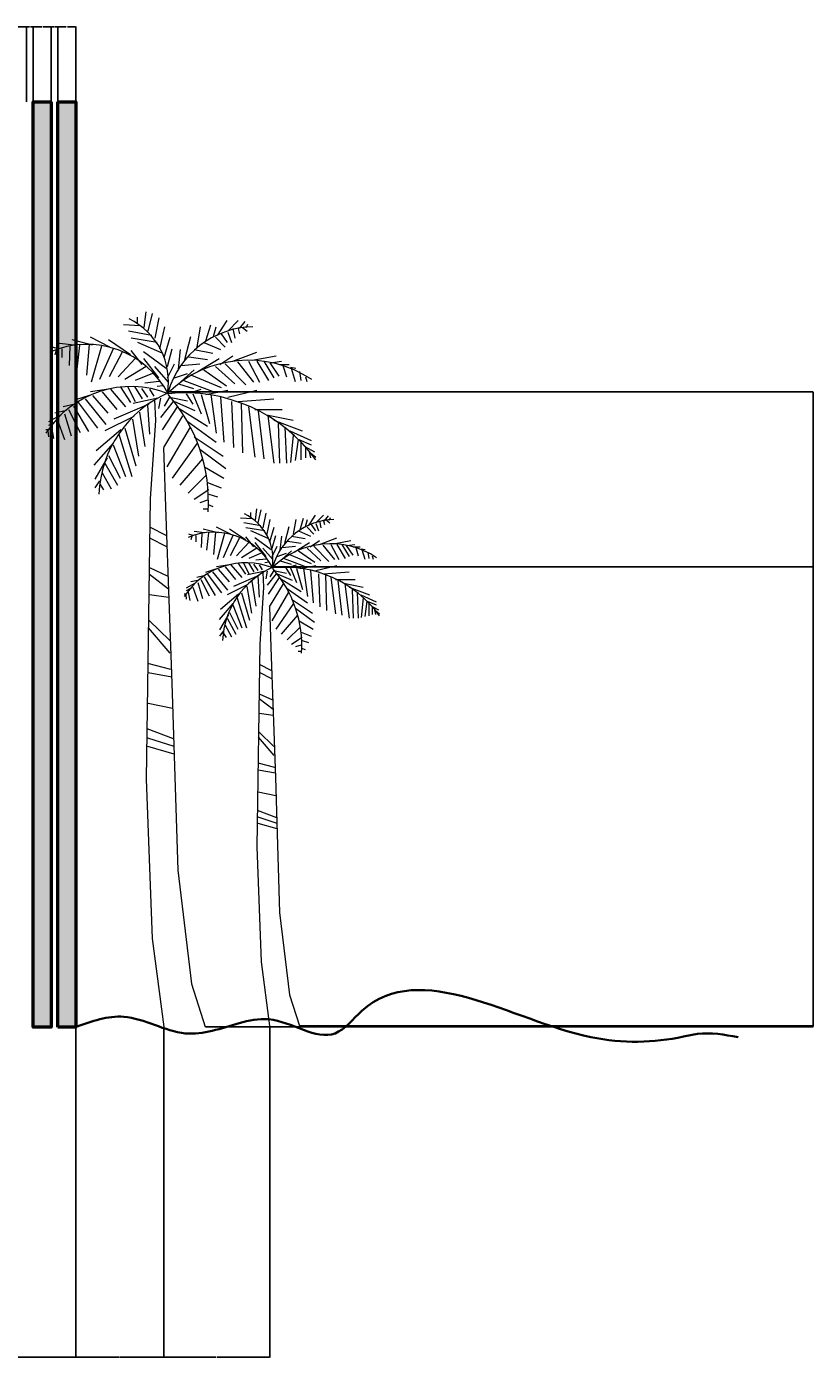
# Model space of a CAD drawing. Units: inches. Extents: x -97 to 1206, y -378 to 680.
# Tile 6 of 6: x 581 to 1206, y -378 to 680. Entities that reach past the tile are written whole.
import ezdxf

# ---------------------------------------------------------------- set-up
doc = ezdxf.new("R2010")
doc.units = ezdxf.units.IN
doc.header["$MEASUREMENT"] = 0
for name, color, linetype, lineweight in [('A-ANNO-DIMS', 2, 'Continuous', 18), ('A-WALL', 7, 'Continuous', 50), ('A-WALL-PATT', 8, 'Continuous', 18), ('C-TOPO', 8, 'Continuous', 35), ('L-PLNT', 82, 'Continuous', 13)]:
    doc.layers.add(name, color=color, linetype=linetype, lineweight=lineweight)
doc.styles.get("Standard").update_dxf_attribs({"font": 'arial.ttf'})
doc.dimstyles.get("Standard").update_dxf_attribs({"dimtxt": 0.18, "dimasz": 0.18, "dimexe": 0.18, "dimexo": 0.0625, "dimgap": 0.09, "dimtad": 0, "dimtih": 1, "dimtoh": 1, "dimdec": 4, "dimzin": 0, "dimdsep": 46, "dimtxsty": 'Standard', "dimcen": 0.09, "dimadec": 0, "dimazin": 0, "dimtfac": 1, "dimtdec": 4, "dimtofl": 0, "dimtmove": 0, "dimatfit": 3, "dimfxl": 1, "dimtolj": 1, "dimtzin": 0, "dimarcsym": 0})
pattern_1 = [(228.0128, (-174.969, -144.922), (-376, -423), [6.3232, -625.9971]), (184.96974, (-179.199, -149.622), (564, 47), [10.8508, -1074.2285]), (132.51045, (-190.009, -150.562), (470, -517), [7.651, -757.4535]), (267.2737, (-208.339, -162.312), (47, 940), [9.8812, -978.2372]), (292.83365, (-208.809, -172.182), (-235, 564), [9.6893, -959.2405]), (357.2737, (-205.049, -181.112), (-940, 47), [9.8812, -978.2372]), (37.69424, (-195.179, -181.582), (-611, -470), [13.0674, -1293.6679]), (72.25533, (-184.839, -173.592), (329, 1034), [12.3369, -1221.3571]), (121.42957, (-181.079, -161.842), (-376, 611), [9.9146, -981.5514]), (175.23636, (-186.249, -153.382), (517, -47), [11.3191, -554.6358]), (222.39744, (-197.5289, -152.442), (-564, -517), [14.63806, -1449.1686]), (138.81407, (-161.809, -162.782), (-329, 282), [4.9961, -494.6207]), (171.46923, (-165.569, -159.492), (611, -94), [9.5051, -941.011]), (225, (-174.97, -158.082), (-5e-15, -47), [6.6468, -59.8213]), (203.1986, (-178.259, -152.442), (235, 94), [3.5794, -354.3619]), (291.8014, (-181.549, -153.852), (-47, 141), [5.062, -248.0407]), (30.96376, (-179.669, -158.552), (141, 94), [8.2217, -265.833]), (161.565, (-172.619, -154.322), (94, -47), [5.945, -142.682]), (16.38954, (-208.809, -153.852), (470, 141), [8.3284, -824.5137]), (70.34618, (-200.819, -151.502), (-188, -517), [6.9871, -691.7182]), (293.1986, (-172.619, -144.922), (-94, 235), [7.1588, -350.7825]), (343.61046, (-169.799, -151.502), (-470, 141), [8.3284, -824.5137]), (339.44395, (-208.809, -182.992), (-235, 94), [8.0314, -393.5368]), (294.77514, (-201.289, -185.812), (-235, 517), [6.7294, -666.2082]), (66.8014, (-172.149, -191.922), (94, 235), [7.1588, -350.7825]), (17.35402, (-169.329, -185.342), (-611, -188), [7.8787, -779.9849]), (69.44395, (-195.179, -191.922), (-94, -235), [4.0157, -397.5525]), (101.3099, (-174.969, -191.922), (-47, 188), [2.3965, -237.2574]), (165.9638, (-175.439, -189.572), (141, -47), [9.6893, -184.0967]), (186.009, (-184.839, -187.222), (470, 47), [8.9794, -888.9544]), (303.6901, (-179.669, -162.782), (-47, 94), [6.7784, -162.6825]), (353.15723, (-175.909, -168.422), (799, -94), [11.8343, -1171.5954]), (60.9454, (-164.159, -169.832), (-188, -329), [4.839, -479.0557]), (90, (-161.81, -165.6), (-47, 47), [2.82, -44.18]), (120.25644, (-185.779, -185.812), (188, -329), [6.5294, -646.4154]), (48.0128, (-189.069, -180.172), (376, 423), [12.6464, -619.674]), (0, (-180.61, -170.77), (47, 47), [12.22, -34.78]), (325.30485, (-168.389, -170.772), (470, -329), [7.4314, -735.7039]), (254.0546, (-162.279, -175.002), (-47, -188), [6.8433, -335.3219]), (207.64598, (-164.159, -181.582), (-893, -470), [11.1421, -1103.0653]), (175.42608, (-174.029, -186.752), (-611, 47), [11.7876, -1166.96645])]

# ---------------------------------------------------------------- blocks, each defined once
blk = doc.blocks.new('*U4')
for p, q in [((-7.5, 199.68), (-7.5, 197.946)), ((-5.567, 196.707), (-4.987, 201.167)), ((-4.407, 195.716), (-3.247, 200.672)), ((-2.474, 193.733), (-1.315, 199.433)), ((15.116, 194.477), (17.822, 198.689)), ((18.015, 195.716), (20.914, 198.689)), ((-6.727, 197.202), (-11.366, 197.45)), ((-3.441, 194.477), (-10.013, 195.716)), ((-1.121, 190.759), (0.232, 196.955)), ((9.317, 191.255), (10.283, 196.955)), ((11.829, 192.99), (13.182, 197.45)), ((13.956, 194.229), (14.729, 196.955)), ((16.082, 194.972), (17.822, 192.494)), ((18.015, 195.468), (18.981, 192.494)), ((19.368, 196.459), (19.948, 193.733)), ((20.914, 196.459), (21.301, 194.972)), ((21.301, 196.459), (22.847, 198.441)), ((22.074, 196.707), (23.427, 195.716)), ((23.234, 196.707), (23.62, 197.698)), ((-29.729, 190.759), (-31.469, 191.255)), ((-25.283, 191.751), (-29.342, 192.246)), ((-26.443, 191.503), (-26.636, 186.051)), ((-20.064, 191.751), (-25.863, 193.238)), ((-23.737, 191.751), (-24.51, 185.06)), ((-21.031, 191.998), (-21.804, 183.325)), ((-15.232, 191.255), (-20.644, 193.981)), ((-17.551, 191.503), (-20.451, 181.343)), ((-9.433, 189.025), (-15.618, 193.238)), ((-1.894, 192.494), (-9.24, 193.733)), ((-0.541, 189.52), (-7.307, 192.494)), ((0.038, 188.281), (1.778, 193.981)), ((5.837, 187.786), (7.577, 194.229)), ((11.25, 192.494), (15.889, 190.512)), ((14.536, 193.981), (17.242, 191.255)), ((-30.309, 190.512), (-30.695, 189.025)), ((-28.763, 190.759), (-28.763, 188.281)), ((-14.265, 190.759), (-18.131, 182.086)), ((-11.753, 189.768), (-15.425, 182.83)), ((-8.08, 188.034), (-12.912, 182.83)), ((-6.147, 186.299), (-9.24, 190.264)), ((-5.76, 190.016), (0.618, 185.308)), ((-5.76, 188.034), (-1.508, 182.582)), ((1.005, 185.803), (2.358, 190.759)), ((4.098, 185.06), (4.678, 190.512)), ((6.997, 188.529), (12.216, 187.786)), ((8.544, 190.512), (13.763, 189.52)), ((9.51, 184.317), (15.502, 188.034)), ((15.695, 186.299), (19.368, 188.777)), ((19.368, 187.29), (26.133, 189.768)), ((23.814, 187.29), (26.907, 181.343)), ((24.78, 187.538), (31.546, 188.777)), ((26.133, 187.29), (29.419, 181.838)), ((28.066, 187.29), (30.966, 182.582)), ((29.999, 186.795), (33.092, 187.29)), ((-4.987, 185.803), (-10.979, 182.086)), ((-3.247, 183.821), (-8.08, 181.838)), ((-2.668, 185.803), (1.198, 181.343)), ((1.005, 182.582), (2.938, 186.547)), ((2.938, 182.582), (6.61, 183.821)), ((4.871, 186.051), (10.09, 186.547)), ((4.871, 181.591), (8.544, 184.812)), ((11.25, 184.812), (17.628, 180.352)), ((14.536, 185.803), (19.948, 180.847)), ((17.242, 186.547), (23.041, 180.599)), ((20.721, 187.042), (25.167, 181.343)), ((29.806, 186.795), (32.319, 183.078)), ((32.512, 186.299), (35.218, 186.299)), ((33.479, 186.051), (34.445, 182.83)), ((35.605, 185.556), (37.151, 185.308)), ((35.798, 185.308), (36.958, 181.591)), ((38.118, 184.317), (38.504, 181.838)), ((-12.332, 180.104), (-9.433, 175.643)), ((-10.206, 180.104), (-8.08, 175.891)), ((-8.273, 180.104), (-6.147, 176.635)), ((-1.315, 181.591), (-5.374, 181.095)), ((-0.348, 180.352), (-1.894, 180.104)), ((4.098, 180.847), (8.35, 179.608)), ((5.644, 181.838), (13.569, 178.865)), ((7.77, 183.325), (16.082, 179.856)), ((39.857, 182.83), (40.244, 181.591)), ((-21.031, 177.626), (-24.897, 176.387)), ((-22.191, 176.635), (-16.391, 169.448)), ((-15.618, 179.36), (-20.644, 178.617)), ((-20.064, 177.626), (-15.812, 172.67)), ((-17.358, 178.617), (-13.299, 173.661)), ((-15.038, 179.36), (-10.786, 174.404)), ((-1.701, 176.882), (-8.66, 175.396)), ((-6.34, 179.608), (-4.6, 177.13)), ((-4.021, 179.36), (-2.861, 177.378)), ((-2.668, 176.387), (-2.376, 170.594)), ((-0.928, 176.882), (-1.508, 173.909)), ((1.585, 177.13), (0.038, 174.652)), ((1.585, 177.13), (6.61, 176.139)), ((6.224, 178.121), (8.157, 175.148)), ((7.384, 178.369), (10.476, 179.36)), ((8.157, 178.121), (10.476, 172.422)), ((10.476, 177.874), (12.796, 169.696)), ((11.829, 177.874), (18.015, 179.113)), ((13.182, 177.874), (14.729, 166.97)), ((15.889, 177.13), (16.855, 164.492)), ((18.015, 177.13), (26.133, 179.113)), ((20.914, 175.891), (30.966, 176.635)), ((-27.409, 173.413), (-30.695, 172.67)), ((-25.09, 175.148), (-28.376, 174.404)), ((-27.989, 172.422), (-26.056, 166.227)), ((-26.829, 173.661), (-23.544, 167.218)), ((-25.476, 174.652), (-21.224, 167.466)), ((-24.317, 175.891), (-18.711, 168.457)), ((-4.214, 175.148), (-14.072, 170.935)), ((-6.92, 172.917), (-5.374, 163.253)), ((-4.6, 174.9), (-4.021, 166.722)), ((2.551, 175.891), (-0.928, 171.431)), ((3.711, 174.404), (-0.541, 167.961)), ((2.938, 175.891), (8.737, 173.413)), ((4.291, 173.909), (12.216, 168.953)), ((18.981, 175.891), (19.561, 163.005)), ((21.688, 175.396), (22.074, 161.518)), ((23.814, 174.404), (25.554, 160.279)), ((25.554, 173.661), (33.285, 173.661)), ((26.52, 173.165), (28.066, 159.784)), ((-28.956, 172.174), (-32.435, 170.192)), ((-31.082, 169.944), (-32.435, 169.2)), ((-31.662, 168.705), (-31.082, 165.483)), ((-29.922, 170.687), (-27.989, 165.235)), ((-8.466, 171.678), (-16.585, 167.713)), ((-8.853, 170.935), (-7.113, 160.527)), ((5.257, 171.926), (-0.155, 163.005)), ((7.384, 168.705), (0.812, 157.553)), ((6.417, 170.439), (14.729, 164.492)), ((28.839, 172.174), (36.378, 170.687)), ((29.226, 171.926), (30.966, 158.545)), ((30.966, 170.687), (38.891, 167.713)), ((32.126, 169.696), (32.512, 158.545)), ((34.058, 168.705), (34.445, 158.545)), ((-32.628, 167.961), (-33.208, 167.961)), ((-32.628, 167.713), (-32.435, 165.979)), ((-12.139, 167.961), (-19.098, 162.014)), ((-12.719, 166.722), (-9.046, 154.828)), ((-10.979, 168.457), (-7.887, 157.801)), ((8.544, 165.979), (16.662, 160.527)), ((35.412, 167.713), (41.404, 164.988)), ((36.378, 166.474), (35.605, 158.792)), ((37.731, 165.235), (36.958, 159.288)), ((37.924, 165.235), (41.404, 163.749)), ((-14.265, 164.244), (-19.678, 158.049)), ((-14.265, 163.749), (-10.786, 154.828)), ((9.317, 164.244), (2.358, 154.332)), ((10.09, 162.51), (17.435, 157.058)), ((38.504, 164.492), (38.504, 159.536)), ((39.664, 163.253), (42.37, 161.766)), ((39.857, 162.757), (39.857, 160.031)), ((40.824, 161.766), (41.21, 160.031)), ((41.21, 161.518), (42.757, 160.279)), ((-16.005, 160.031), (-19.484, 154.084)), ((-16.585, 158.545), (-13.106, 152.35)), ((-15.618, 160.775), (-12.332, 154.332)), ((10.863, 159.784), (4.484, 152.35)), ((11.443, 157.553), (16.855, 154.332)), ((-18.131, 153.589), (-19.484, 151.606)), ((-17.358, 155.819), (-14.845, 151.358)), ((11.829, 155.075), (6.804, 150.119)), ((-17.938, 152.597), (-16.972, 151.111)), ((12.603, 151.111), (8.544, 148.385)), ((12.216, 153.093), (16.082, 151.606)), ((12.603, 149.872), (15.116, 149.128)), ((12.216, 148.137), (10.09, 147.393)), ((12.409, 146.898), (13.763, 146.402)), ((12.409, 145.659), (11.056, 145.659)), ((-4.081, 140.645), (0.753, 138.261)), ((-4.081, 137.547), (0.753, 135.163)), ((-4.081, 129.205), (1.124, 126.821)), ((-4.081, 127.298), (1.31, 123.246)), ((-4.081, 121.578), (1.31, 120.863)), ((-4.267, 114.428), (1.682, 108.708)), ((-4.453, 112.283), (1.682, 105.133)), ((-4.639, 102.273), (1.868, 100.604)), ((-4.453, 99.651), (2.24, 98.459)), ((-4.453, 91.071), (2.426, 89.641)), ((-4.825, 83.921), (2.612, 81.061)), ((-4.639, 81.299), (2.797, 78.916)), ((-4.639, 78.916), (2.797, 76.771))]:
    blk.add_line(p, q)
for points in [[(-2.363, 170.553), (-3.88, 148.505), (-4.988, 69.634), (-3.325, 24.869), (0, 0)], [(-0.116, 162.848), (0.554, 143.532), (2.217, 96.635), (3.88, 44.054), (7.76, 12.079), (11.64, 0)]]:
    blk.add_lwpolyline(points)
for centre, radius, start, end in [((-18.427, 181.448), 19.715, 350.285, 64.11229), ((25.595, 171.567), 25.395, 91.40319, 163.882), ((-21.738, 166.094), 25.899, 27.67115, 112.5305), ((23.687, 155.341), 32.188, 56.19272, 134.3213), ((-9.259, 151.732), 28.386, 68.38311, 147.5322), ((14.394, 148.393), 32.752, 113.7592, 177.4133), ((5.828, 132.718), 45.639, 35.98777, 95.82273), ((-32.8, 147.923), 45.309, 356.1943, 41.37848)]:
    blk.add_arc(centre, radius, start, end)
blk = doc.blocks.new('*D11')
at = {"layer": 'A-ANNO-DIMS', "color": 0, "lineweight": -2, "transparency": 16777216}
for p, q in [((-36.9, -115.2), (-36.9, -377.6)), ((620.2, -115.2), (620.2, -377.6)), ((-36.7, -377.4), (291.3, -377.4)), ((620, -377.4), (292, -377.4))]:
    blk.add_line(p, q, dxfattribs=at)
at = {"layer": 'A-ANNO-DIMS', "color": 0, "transparency": 16777216}
for points in [[(-36.7, -377.4), (-36.7, -377.4), (-36.9, -377.4)], [(620, -377.4), (620, -377.4), (620.2, -377.4)]]:
    blk.add_solid(points, dxfattribs=at)
at = {"layer": 'Defpoints', "color": 0, "transparency": 16777216}
for p in [(-36.9, -115.1), (620.2, -115.1), (620.2, -377.4)]:
    blk.add_point(p, dxfattribs=at)
at = {"layer": 'A-ANNO-DIMS', "color": 0, "transparency": 16777216, "insert": (291.6, -377.4), "char_height": 0.18, "attachment_point": 5}
blk.add_mtext('\\A1;657.1', dxfattribs=at)
blk = doc.blocks.new('*D22')
at = {"layer": 'A-ANNO-DIMS', "color": 0, "lineweight": -2, "transparency": 16777216}
for p, q in [((523.9, 619.9), (523.9, 679.5)), ((524.1, 679.4), (552.2, 679.4)), ((581, 679.4), (553, 679.4)), ((581.2, 619.9), (581.2, 679.5))]:
    blk.add_line(p, q, dxfattribs=at)
at = {"layer": 'A-ANNO-DIMS', "color": 0, "transparency": 16777216}
for points in [[(524.1, 679.4), (524.1, 679.3), (523.9, 679.4)], [(581, 679.4), (581, 679.3), (581.2, 679.4)]]:
    blk.add_solid(points, dxfattribs=at)
at = {"layer": 'Defpoints', "color": 0, "transparency": 16777216}
for p in [(581.2, 679.4), (523.9, 619.9), (581.2, 619.9)]:
    blk.add_point(p, dxfattribs=at)
at = {"layer": 'A-ANNO-DIMS', "color": 0, "transparency": 16777216, "insert": (552.6, 679.4), "char_height": 0.18, "attachment_point": 5}
blk.add_mtext('\\A1;57.28', dxfattribs=at)
blk = doc.blocks.new('*D23')
at = {"layer": 'A-ANNO-DIMS', "color": 0, "lineweight": -2, "transparency": 16777216}
for p, q in [((581.2, 619.9), (581.2, 679.5)), ((581.4, 679.4), (583.6, 679.4)), ((586.4, 679.4), (584.2, 679.4)), ((586.5, 619.9), (586.5, 679.5))]:
    blk.add_line(p, q, dxfattribs=at)
at = {"layer": 'A-ANNO-DIMS', "color": 0, "transparency": 16777216}
for points in [[(581.4, 679.4), (581.4, 679.3), (581.2, 679.4)], [(586.4, 679.4), (586.4, 679.3), (586.5, 679.4)]]:
    blk.add_solid(points, dxfattribs=at)
at = {"layer": 'Defpoints', "color": 0, "transparency": 16777216}
for p in [(586.5, 679.4), (581.2, 619.9), (586.5, 619.9)]:
    blk.add_point(p, dxfattribs=at)
at = {"layer": 'A-ANNO-DIMS', "color": 0, "transparency": 16777216, "insert": (583.9, 679.4), "char_height": 0.18, "attachment_point": 5}
blk.add_mtext('\\A1;5.33', dxfattribs=at)
blk = doc.blocks.new('*D24')
at = {"layer": 'A-ANNO-DIMS', "color": 0, "lineweight": -2, "transparency": 16777216}
for p, q in [((586.5, 619.9), (586.5, 679.5)), ((586.7, 679.4), (593.2, 679.4)), ((600.5, 679.4), (594.1, 679.4)), ((600.7, 619.9), (600.7, 679.5))]:
    blk.add_line(p, q, dxfattribs=at)
at = {"layer": 'A-ANNO-DIMS', "color": 0, "transparency": 16777216}
for points in [[(586.7, 679.4), (586.7, 679.3), (586.5, 679.4)], [(600.5, 679.4), (600.5, 679.3), (600.7, 679.4)]]:
    blk.add_solid(points, dxfattribs=at)
at = {"layer": 'Defpoints', "color": 0, "transparency": 16777216}
for p in [(600.7, 679.4), (586.5, 619.9), (600.7, 619.9)]:
    blk.add_point(p, dxfattribs=at)
at = {"layer": 'A-ANNO-DIMS', "color": 0, "transparency": 16777216, "insert": (593.6, 679.4), "char_height": 0.18, "attachment_point": 5}
blk.add_mtext('\\A1;14.158', dxfattribs=at)
blk = doc.blocks.new('*D25')
at = {"layer": 'A-ANNO-DIMS', "color": 0, "lineweight": -2, "transparency": 16777216}
for p, q in [((600.7, 619.9), (600.7, 679.5)), ((600.9, 679.4), (603, 679.4)), ((605.8, 679.4), (603.7, 679.4)), ((606, 619.9), (606, 679.5))]:
    blk.add_line(p, q, dxfattribs=at)
at = {"layer": 'A-ANNO-DIMS', "color": 0, "transparency": 16777216}
for points in [[(600.9, 679.4), (600.9, 679.3), (600.7, 679.4)], [(605.8, 679.4), (605.8, 679.3), (606, 679.4)]]:
    blk.add_solid(points, dxfattribs=at)
at = {"layer": 'Defpoints', "color": 0, "transparency": 16777216}
for p in [(606, 679.4), (600.7, 619.9), (606, 619.9)]:
    blk.add_point(p, dxfattribs=at)
at = {"layer": 'A-ANNO-DIMS', "color": 0, "transparency": 16777216, "insert": (603.4, 679.4), "char_height": 0.18, "attachment_point": 5}
blk.add_mtext('\\A1;5.33', dxfattribs=at)
blk = doc.blocks.new('*D26')
at = {"layer": 'A-ANNO-DIMS', "color": 0, "lineweight": -2, "transparency": 16777216}
for p, q in [((606, 619.9), (606, 679.5)), ((606.2, 679.4), (612.7, 679.4)), ((620, 679.4), (613.6, 679.4)), ((620.2, 619.9), (620.2, 679.5))]:
    blk.add_line(p, q, dxfattribs=at)
at = {"layer": 'A-ANNO-DIMS', "color": 0, "transparency": 16777216}
for points in [[(606.2, 679.4), (606.2, 679.3), (606, 679.4)], [(620, 679.4), (620, 679.3), (620.2, 679.4)]]:
    blk.add_solid(points, dxfattribs=at)
at = {"layer": 'Defpoints', "color": 0, "transparency": 16777216}
for p in [(620.2, 679.4), (606, 619.9), (620.2, 619.9)]:
    blk.add_point(p, dxfattribs=at)
at = {"layer": 'A-ANNO-DIMS', "color": 0, "transparency": 16777216, "insert": (613.1, 679.4), "char_height": 0.18, "attachment_point": 5}
blk.add_mtext('\\A1;14.158', dxfattribs=at)
blk = doc.blocks.new('*D27')
at = {"layer": 'A-ANNO-DIMS', "color": 0, "lineweight": -2, "transparency": 16777216}
for p, q in [((620.2, -115.2), (620.2, -377.6)), ((690.3, -115), (690.3, -377.6)), ((620.4, -377.4), (654.9, -377.4)), ((690.1, -377.4), (655.5, -377.4))]:
    blk.add_line(p, q, dxfattribs=at)
at = {"layer": 'A-ANNO-DIMS', "color": 0, "transparency": 16777216}
for points in [[(620.4, -377.4), (620.4, -377.4), (620.2, -377.4)], [(690.1, -377.4), (690.1, -377.4), (690.3, -377.4)]]:
    blk.add_solid(points, dxfattribs=at)
at = {"layer": 'Defpoints', "color": 0, "transparency": 16777216}
for p in [(620.2, -115.1), (690.3, -115), (690.3, -377.4)]:
    blk.add_point(p, dxfattribs=at)
at = {"layer": 'A-ANNO-DIMS', "color": 0, "transparency": 16777216, "insert": (655.2, -377.4), "char_height": 0.18, "attachment_point": 5}
blk.add_mtext('\\A1;70.1', dxfattribs=at)
blk = doc.blocks.new('*D28')
at = {"layer": 'A-ANNO-DIMS', "color": 0, "lineweight": -2, "transparency": 16777216}
for p, q in [((690.3, -115), (690.3, -377.6)), ((774.3, -114.4), (774.3, -377.6)), ((690.5, -377.4), (731.9, -377.4)), ((774.1, -377.4), (732.7, -377.4))]:
    blk.add_line(p, q, dxfattribs=at)
at = {"layer": 'A-ANNO-DIMS', "color": 0, "transparency": 16777216}
for points in [[(690.5, -377.4), (690.5, -377.4), (690.3, -377.4)], [(774.1, -377.4), (774.1, -377.4), (774.3, -377.4)]]:
    blk.add_solid(points, dxfattribs=at)
at = {"layer": 'Defpoints', "color": 0, "transparency": 16777216}
for p in [(690.3, -115), (774.3, -114.3), (774.3, -377.4)]:
    blk.add_point(p, dxfattribs=at)
at = {"layer": 'A-ANNO-DIMS', "color": 0, "transparency": 16777216, "insert": (732.3, -377.4), "char_height": 0.18, "attachment_point": 5}
blk.add_mtext('\\A1;83.98', dxfattribs=at)
blk = doc.blocks.new('*D29')
at = {"layer": 'A-ANNO-DIMS', "color": 0, "lineweight": -2, "transparency": 16777216}
for p, q in [((693.7, 389.3), (1206.1, 389.3)), ((1205.9, 389.2), (1205.9, 137.4)), ((1205.9, -114.8), (1205.9, 137)), ((723.2, -115), (1206.1, -115))]:
    blk.add_line(p, q, dxfattribs=at)
at = {"layer": 'A-ANNO-DIMS', "color": 0, "transparency": 16777216}
for points in [[(1205.8, 389.2), (1205.9, 389.2), (1205.9, 389.3)], [(1205.8, -114.8), (1205.9, -114.8), (1205.9, -115)]]:
    blk.add_solid(points, dxfattribs=at)
at = {"layer": 'Defpoints', "color": 0, "transparency": 16777216}
for p in [(693.7, 389.3), (1205.9, 389.3), (723.2, -115)]:
    blk.add_point(p, dxfattribs=at)
at = {"layer": 'A-ANNO-DIMS', "color": 0, "transparency": 16777216, "insert": (1205.9, 137.2), "char_height": 0.18, "attachment_point": 5}
blk.add_mtext('\\A1;504.3', dxfattribs=at)
blk = doc.blocks.new('*D30')
at = {"layer": 'A-ANNO-DIMS', "color": 0, "lineweight": -2, "transparency": 16777216}
for p, q in [((776.8, 250.5), (1206.1, 250.5)), ((1205.9, 250.4), (1205.9, 68.3)), ((1205.9, -114.1), (1205.9, 67.9)), ((798.1, -114.3), (1206.1, -114.3))]:
    blk.add_line(p, q, dxfattribs=at)
at = {"layer": 'A-ANNO-DIMS', "color": 0, "transparency": 16777216}
for points in [[(1205.8, 250.4), (1205.9, 250.4), (1205.9, 250.5)], [(1205.8, -114.1), (1205.9, -114.1), (1205.9, -114.3)]]:
    blk.add_solid(points, dxfattribs=at)
at = {"layer": 'Defpoints', "color": 0, "transparency": 16777216}
for p in [(776.7, 250.5), (1205.9, 250.5), (798.1, -114.3)]:
    blk.add_point(p, dxfattribs=at)
at = {"layer": 'A-ANNO-DIMS', "color": 0, "transparency": 16777216, "insert": (1205.9, 68.1), "char_height": 0.18, "attachment_point": 5}
blk.add_mtext('\\A1;364.8', dxfattribs=at)

msp = doc.modelspace()

# ---------------------------------------------------------------- hatches: boundary and pattern name
at = {"layer": 'A-WALL-PATT'}
h = msp.add_hatch(dxfattribs=at)
h.set_pattern_fill('GRAVEL', color=256, scale=47)
h.set_pattern_definition(pattern_1)
h.paths.add_polyline_path([(600.6973, 619.8552), (586.5391, 619.8552), (586.5391, -115.1448), (600.6973, -115.1448)])
h = msp.add_hatch(dxfattribs=at)
h.set_pattern_fill('GRAVEL', color=256, scale=47)
h.set_pattern_definition(pattern_1)
h.paths.add_polyline_path([(620.1851, 619.8552), (606.027, 619.8552), (606.027, -115.1448), (620.1851, -115.1448)])

# ---------------------------------------------------------------- linework, layer by layer
at = {"layer": 'A-WALL'}
msp.add_lwpolyline([(600.6973, 619.8552), (600.6973, -115.1448), (586.5391, -115.1448), (586.5391, 619.8552)], close=True, dxfattribs=at)
for points in [[(606.027, 619.8552), (620.1851, 619.8552), (620.1851, -115.1448), (606.027, -115.1448)], [(606.027, -115.1448), (606.027, 619.8552)]]:
    msp.add_lwpolyline(points, dxfattribs=at)
at = {"layer": 'C-TOPO'}
msp.add_open_spline([(620.1851, -115.1448), (632.9746, -110.6122), (662.3372, -100.2063), (704.7056, -127.6953), (743.667, -113.2232), (783.1679, -104.1819), (821.3604, -133.7193), (883.2442, -52.6509), (995.0019, -130.0931), (1082.6903, -127.7364), (1120.9658, -118.6183), (1135.5504, -121.255), (1146.3757, -123.2121)], degree=3, knots=[0, 0, 0, 0, 39.055670918, 89.666016789, 133.337314924, 156.934893283, 210.787525561, 238.52559643, 421.7403402, 495.257771352, 506.508523833, 538.904961114, 538.904961114, 538.904961114, 538.904961114], dxfattribs=at)

# ---------------------------------------------------------------- block references
at = {"layer": 'L-PLNT'}
for p, xscale, yscale, zscale in [((690.2914, -114.9517), 2.823339693315601, 2.823339693315601, 2.823339693315601), ((774.2758, -114.2996), 2.042538135110552, 2.042538135110552, 2.042538135110552)]:
    msp.add_blockref('*U4', p, dxfattribs=dict(at, xscale=xscale, yscale=yscale, zscale=zscale))

# ---------------------------------------------------------------- dimensions: what is measured, and where the dimension line sits
at = {"layer": 'A-ANNO-DIMS'}
for base, p1, p2, override, picture, middle in [((581.2095, 679.3552), (523.9261, 619.8552), (581.2095, 619.8552), {"dimdec": 2, "dimlfac": 1, "dimrnd": 0, "dimzin": 0, "dimdsep": 46, "dimlunit": 2}, '*D22', (552.5678, 679.3552)), ((586.5391, 679.3552), (581.2095, 619.8552), (586.5391, 619.8552), {"dimdec": 2, "dimlfac": 1, "dimrnd": 0, "dimzin": 0, "dimdsep": 46, "dimlunit": 2}, '*D23', (583.8743, 679.3552)), ((600.6973, 679.3552), (586.5391, 619.8552), (600.6973, 619.8552), {"dimdec": 3, "dimlfac": 1, "dimrnd": 0, "dimzin": 0, "dimdsep": 46, "dimlunit": 2}, '*D24', (593.6182, 679.3552)), ((606.027, 679.3552), (600.6973, 619.8552), (606.027, 619.8552), {"dimdec": 2, "dimlfac": 1, "dimrnd": 0, "dimzin": 0, "dimdsep": 46, "dimlunit": 2}, '*D25', (603.3621, 679.3552)), ((620.1851, 679.3552), (606.027, 619.8552), (620.1851, 619.8552), {"dimdec": 3, "dimlfac": 1, "dimrnd": 0, "dimzin": 0, "dimdsep": 46, "dimlunit": 2}, '*D26', (613.1061, 679.3552)), ((620.1851, -377.4132), (-36.9051, -115.1448), (620.1851, -115.1448), {"dimdec": 1, "dimlfac": 1, "dimrnd": 0, "dimzin": 0, "dimdsep": 46, "dimlunit": 2}, '*D11', (291.64, -377.4132)), ((690.2914, -377.4132), (620.1851, -115.1448), (690.2914, -114.9517), {"dimdec": 1, "dimlfac": 1, "dimrnd": 0, "dimzin": 0, "dimdsep": 46, "dimlunit": 2}, '*D27', (655.2383, -377.4132)), ((774.2758, -377.4132), (690.2914, -114.9517), (774.2758, -114.2996), {"dimdec": 2, "dimlfac": 1, "dimrnd": 0, "dimzin": 0, "dimdsep": 46, "dimlunit": 2}, '*D28', (732.2836, -377.4132))]:
    dim = msp.add_linear_dim(base=base, p1=p1, p2=p2, dimstyle='Standard', override=override, dxfattribs=at)
    dim.commit()
    dim.dimension.update_dxf_attribs({"geometry": picture, "text_midpoint": middle})
for base, p1, p2, picture, middle in [((1205.8757, 389.3453), (723.1551, -114.9517), (693.6733, 389.3453), '*D29', (1205.8757, 137.1968)), ((1205.8757, 250.5328), (798.0509, -114.2996), (776.7224, 250.5328), '*D30', (1205.8757, 68.1166))]:
    dim = msp.add_linear_dim(base=base, p1=p1, p2=p2, angle=90, dimstyle='Standard', override={"dimdec": 1, "dimlfac": 1, "dimrnd": 0, "dimzin": 0, "dimdsep": 46, "dimlunit": 2}, dxfattribs=at)
    dim.commit()
    dim.dimension.update_dxf_attribs({"geometry": picture, "text_midpoint": middle})

doc.saveas('drawing.dxf')
